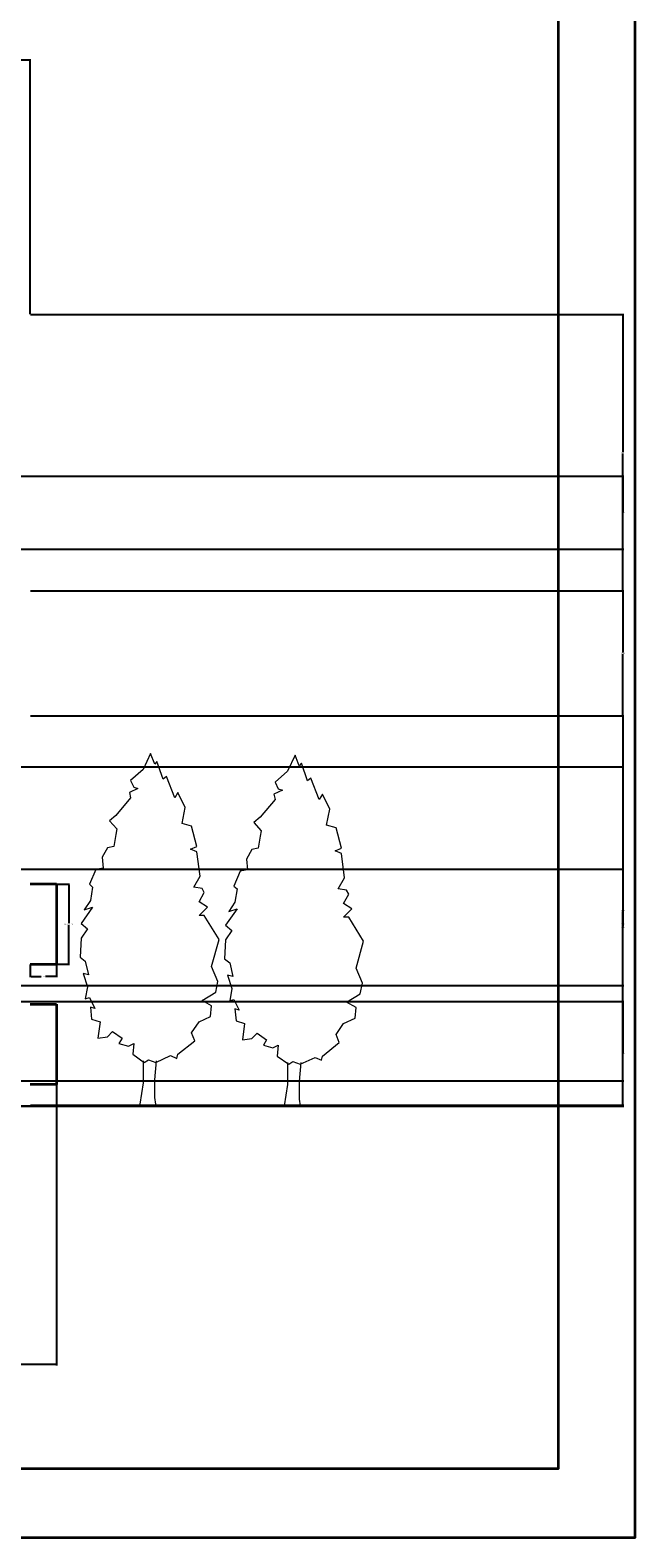
# Model space of a CAD drawing. Units: inches. Extents: x -279 to 364, y -385 to 335.
# Tile 4 of 9: x 238 to 364, y -385 to -72. Entities that reach past the tile are written whole.
import ezdxf

# ---------------------------------------------------------------- set-up
doc = ezdxf.new("R2010")
doc.units = ezdxf.units.IN
doc.header["$MEASUREMENT"] = 0
for name, color, linetype, lineweight in [('A-ANNO-DIMS', 2, 'Continuous', 18), ('A-ANNO-TTLB', 7, 'Continuous', 35), ('A-WALL', 7, 'Continuous', 35), ('C-TOPO', 32, 'Continuous', 30), ('L-PLNT', 94, 'Continuous', 13)]:
    doc.layers.add(name, color=color, linetype=linetype, lineweight=lineweight)
doc.styles.get("Standard").update_dxf_attribs({"font": 'arial.ttf'})
doc.dimstyles.get("Standard").update_dxf_attribs({"dimtxt": 0.18, "dimasz": 0.18, "dimexe": 0.18, "dimexo": 0.0625, "dimgap": 0.09, "dimtad": 0, "dimtih": 1, "dimtoh": 1, "dimdec": 4, "dimzin": 0, "dimdsep": 46, "dimtxsty": 'Standard', "dimcen": 0.09, "dimadec": 0, "dimazin": 0, "dimtfac": 1, "dimtdec": 4, "dimtofl": 0, "dimtmove": 0, "dimatfit": 3, "dimfxl": 1, "dimtolj": 1, "dimtzin": 0, "dimarcsym": 0})

# ---------------------------------------------------------------- blocks, each defined once
blk = doc.blocks.new('*U3')
blk.add_lwpolyline([(-2.754, 191.699), (-6.78, 182.851), (-13.682, 176.953), (-11.956, 173.266), (-9.656, 172.529), (-14.257, 170.317), (-13.682, 167.368), (-21.733, 157.783), (-25.184, 154.834), (-21.158, 150.41), (-21.733, 147.461), (-22.884, 140.825), (-26.334, 140.087), (-29.21, 134.926), (-28.635, 129.028), (-32.661, 128.291), (-36.111, 120.18), (-34.386, 118.706), (-35.536, 111.333), (-38.987, 106.171), (-34.386, 107.646), (-40.712, 98.798), (-37.261, 95.849), (-40.712, 90.688), (-41.287, 80.366), (-38.412, 78.154), (-36.686, 70.781), (-39.562, 71.518), (-37.261, 64.145), (-38.412, 57.509), (-36.111, 58.247), (-33.236, 52.348), (-35.536, 53.086), (-34.961, 46.45), (-30.36, 44.975), (-31.51, 36.128), (-26.334, 36.865), (-23.459, 39.814), (-18.283, 36.128), (-20.008, 33.178), (-14.832, 31.704), (-11.956, 33.178), (-12.531, 27.28), (-6.205, 22.856), (-3.905, 24.331), (0.121, 22.856), (8.173, 26.543), (11.624, 25.068), (12.199, 27.28), (21.4, 34.653), (19.675, 39.077), (23.701, 44.975), (30.027, 47.924), (30.602, 53.823), (25.426, 56.772), (32.903, 61.196), (34.053, 67.094), (30.602, 75.205), (34.628, 89.951), (26.576, 103.222), (23.701, 103.222), (28.302, 107.646), (23.701, 110.595), (26.576, 115.756), (25.426, 117.968), (20.825, 118.706), (24.276, 124.604), (22.551, 137.876), (19.1, 139.35), (22.551, 140.825), (19.675, 151.884), (14.499, 153.359), (16.224, 162.207), (12.199, 170.317), (10.473, 167.368), (5.872, 179.165), (4.147, 177.69), (0.696, 187.275), (-0.454, 185.8)], close=True)
for points in [[(-6.813, 23.669), (-6.813, 11.669), (-8.627, 0)], [(0.387, 23.669), (-0.576, 13.271), (-0.576, 3.686), (0, 0)]]:
    blk.add_lwpolyline(points)
blk = doc.blocks.new('PROJECTION-SIDE')
for p, q in [((0, 16.72), (5.49, 16.72)), ((5.49, 16.72), (5.49, 0)), ((5.49, 0), (0, 0))]:
    blk.add_line(p, q)
blk = doc.blocks.new('*D68')
at = {"layer": 'A-ANNO-DIMS', "color": 0, "lineweight": -2, "transparency": 16777216}
for p, q in [((243.89, -249.21), (246.52, -249.21)), ((246.34, -249.39), (246.34, -257.38)), ((246.34, -265.74), (246.34, -257.75)), ((243.89, -265.92), (246.52, -265.92))]:
    blk.add_line(p, q, dxfattribs=at)
at = {"layer": 'A-ANNO-DIMS', "color": 0, "transparency": 16777216}
for points in [[(246.31, -249.39), (246.37, -249.39), (246.34, -249.21)], [(246.31, -265.74), (246.37, -265.74), (246.34, -265.92)]]:
    blk.add_solid(points, dxfattribs=at)
at = {"layer": 'Defpoints', "color": 0, "transparency": 16777216}
for p in [(243.83, -249.21), (246.34, -249.21), (243.83, -265.92)]:
    blk.add_point(p, dxfattribs=at)
at = {"layer": 'A-ANNO-DIMS', "color": 0, "transparency": 16777216, "insert": (246.34, -257.56), "char_height": 0.18, "attachment_point": 5}
blk.add_mtext('\\A1;RETURN 17 TYP.', dxfattribs=at)
blk = doc.blocks.new('*D69')
at = {"layer": 'A-ANNO-DIMS', "color": 0, "lineweight": -2, "transparency": 16777216}
for p, q in [((238.34, -265.99), (238.34, -268.61)), ((243.83, -265.99), (243.83, -268.61)), ((238.52, -268.43), (240.62, -268.43)), ((243.65, -268.43), (241.54, -268.43))]:
    blk.add_line(p, q, dxfattribs=at)
at = {"layer": 'A-ANNO-DIMS', "color": 0, "transparency": 16777216}
for points in [[(238.52, -268.4), (238.52, -268.46), (238.34, -268.43)], [(243.65, -268.4), (243.65, -268.46), (243.83, -268.43)]]:
    blk.add_solid(points, dxfattribs=at)
at = {"layer": 'Defpoints', "color": 0, "transparency": 16777216}
for p in [(238.34, -265.92), (243.83, -265.92), (243.83, -268.43)]:
    blk.add_point(p, dxfattribs=at)
at = {"layer": 'A-ANNO-DIMS', "color": 0, "transparency": 16777216, "insert": (241.08, -268.43), "char_height": 0.18, "attachment_point": 5}
blk.add_mtext('\\A1;5 TYP.', dxfattribs=at)
blk = doc.blocks.new('*D97')
at = {"layer": 'A-ANNO-DIMS', "color": 0, "lineweight": -2, "transparency": 16777216}
for p, q in [((243.83, -291), (243.83, -349.37)), ((-125.57, -295.46), (-125.57, -349.37)), ((-125.39, -349.19), (58.74, -349.19)), ((243.65, -349.19), (59.52, -349.19))]:
    blk.add_line(p, q, dxfattribs=at)
at = {"layer": 'A-ANNO-DIMS', "color": 0, "transparency": 16777216}
for points in [[(-125.39, -349.16), (-125.39, -349.22), (-125.57, -349.19)], [(243.65, -349.16), (243.65, -349.22), (243.83, -349.19)]]:
    blk.add_solid(points, dxfattribs=at)
at = {"layer": 'Defpoints', "color": 0, "transparency": 16777216}
for p in [(243.83, -290.94), (-125.57, -295.4), (243.83, -349.19)]:
    blk.add_point(p, dxfattribs=at)
at = {"layer": 'A-ANNO-DIMS', "color": 0, "transparency": 16777216, "insert": (59.13, -349.19), "char_height": 0.18, "attachment_point": 5}
blk.add_mtext('\\A1;369.4', dxfattribs=at)
blk = doc.blocks.new('*D101')
at = {"layer": 'A-ANNO-DIMS', "color": 0, "lineweight": -2, "transparency": 16777216}
for p, q in [((114.35, -130.65), (114.35, -77.65)), ((114.53, -77.83), (176.06, -77.83)), ((238.16, -77.83), (176.62, -77.83)), ((238.34, -130.65), (238.34, -77.65))]:
    blk.add_line(p, q, dxfattribs=at)
at = {"layer": 'A-ANNO-DIMS', "color": 0, "transparency": 16777216}
for points in [[(114.53, -77.8), (114.53, -77.86), (114.35, -77.83)], [(238.16, -77.8), (238.16, -77.86), (238.34, -77.83)]]:
    blk.add_solid(points, dxfattribs=at)
at = {"layer": 'Defpoints', "color": 0, "transparency": 16777216}
for p in [(238.34, -77.83), (114.35, -130.71), (238.34, -130.71)]:
    blk.add_point(p, dxfattribs=at)
at = {"layer": 'A-ANNO-DIMS', "color": 0, "transparency": 16777216, "insert": (176.34, -77.83), "char_height": 0.18, "attachment_point": 5}
blk.add_mtext('\\A1;124', dxfattribs=at)
blk = doc.blocks.new('*D102')
at = {"layer": 'A-ANNO-DIMS', "color": 0, "lineweight": -2, "transparency": 16777216}
for p, q in [((238.4, -214.21), (361.74, -214.21)), ((361.56, -214.39), (361.56, -254.55)), ((361.56, -295.07), (361.56, -254.91)), ((238.4, -295.25), (361.74, -295.25))]:
    blk.add_line(p, q, dxfattribs=at)
at = {"layer": 'A-ANNO-DIMS', "color": 0, "transparency": 16777216}
for points in [[(361.53, -214.39), (361.59, -214.39), (361.56, -214.21)], [(361.53, -295.07), (361.59, -295.07), (361.56, -295.25)]]:
    blk.add_solid(points, dxfattribs=at)
at = {"layer": 'Defpoints', "color": 0, "transparency": 16777216}
for p in [(238.34, -214.21), (361.56, -214.21), (238.34, -295.25)]:
    blk.add_point(p, dxfattribs=at)
at = {"layer": 'A-ANNO-DIMS', "color": 0, "transparency": 16777216, "insert": (361.56, -254.73), "char_height": 0.18, "attachment_point": 5}
blk.add_mtext('\\A1;81.04', dxfattribs=at)
blk = doc.blocks.new('*D103')
at = {"layer": 'A-ANNO-DIMS', "color": 0, "lineweight": -2, "transparency": 16777216}
for p, q in [((238.4, -188.22), (361.74, -188.22)), ((361.56, -188.4), (361.56, -201.03)), ((361.56, -214.03), (361.56, -201.4)), ((238.4, -214.21), (361.74, -214.21))]:
    blk.add_line(p, q, dxfattribs=at)
at = {"layer": 'A-ANNO-DIMS', "color": 0, "transparency": 16777216}
for points in [[(361.53, -188.4), (361.59, -188.4), (361.56, -188.22)], [(361.53, -214.03), (361.59, -214.03), (361.56, -214.21)]]:
    blk.add_solid(points, dxfattribs=at)
at = {"layer": 'Defpoints', "color": 0, "transparency": 16777216}
for p in [(238.34, -188.22), (361.56, -188.22), (238.34, -214.21)]:
    blk.add_point(p, dxfattribs=at)
at = {"layer": 'A-ANNO-DIMS', "color": 0, "transparency": 16777216, "insert": (361.56, -201.21), "char_height": 0.18, "attachment_point": 5}
blk.add_mtext('\\A1;25.994', dxfattribs=at)
blk = doc.blocks.new('*D104')
at = {"layer": 'A-ANNO-DIMS', "color": 0, "lineweight": -2, "transparency": 16777216}
for p, q in [((238.4, -130.71), (361.74, -130.71)), ((361.56, -130.89), (361.56, -159.28)), ((361.56, -188.04), (361.56, -159.65)), ((238.4, -188.22), (361.74, -188.22))]:
    blk.add_line(p, q, dxfattribs=at)
at = {"layer": 'A-ANNO-DIMS', "color": 0, "transparency": 16777216}
for points in [[(361.53, -130.89), (361.59, -130.89), (361.56, -130.71)], [(361.53, -188.04), (361.59, -188.04), (361.56, -188.22)]]:
    blk.add_solid(points, dxfattribs=at)
at = {"layer": 'Defpoints', "color": 0, "transparency": 16777216}
for p in [(238.34, -130.71), (361.56, -130.71), (238.34, -188.22)]:
    blk.add_point(p, dxfattribs=at)
at = {"layer": 'A-ANNO-DIMS', "color": 0, "transparency": 16777216, "insert": (361.56, -159.47), "char_height": 0.18, "attachment_point": 5}
blk.add_mtext('\\A1;57.5', dxfattribs=at)
blk = doc.blocks.new('*D111')
at = {"layer": 'A-ANNO-DIMS', "color": 0, "lineweight": -2, "transparency": 16777216}
for p, q in [((184.08, -164.35), (361.74, -164.35)), ((361.56, -164.53), (361.56, -171.76)), ((361.56, -179.35), (361.56, -172.12)), ((184.92, -179.53), (361.74, -179.53))]:
    blk.add_line(p, q, dxfattribs=at)
at = {"layer": 'A-ANNO-DIMS', "color": 0, "transparency": 16777216}
for points in [[(361.53, -164.53), (361.59, -164.53), (361.56, -164.35)], [(361.53, -179.35), (361.59, -179.35), (361.56, -179.53)]]:
    blk.add_solid(points, dxfattribs=at)
at = {"layer": 'Defpoints', "color": 0, "transparency": 16777216}
for p in [(184.01, -164.35), (184.86, -179.53), (361.56, -179.53)]:
    blk.add_point(p, dxfattribs=at)
at = {"layer": 'A-ANNO-DIMS', "color": 0, "transparency": 16777216, "insert": (361.56, -171.94), "char_height": 0.18, "attachment_point": 5}
blk.add_mtext('\\A1;15.182', dxfattribs=at)
blk = doc.blocks.new('*D112')
at = {"layer": 'A-ANNO-DIMS', "color": 0, "lineweight": -2, "transparency": 16777216}
for p, q in [((177.91, -246.11), (361.74, -246.11)), ((361.56, -246.29), (361.56, -258.03)), ((361.56, -270.13), (361.56, -258.39)), ((177.91, -270.31), (361.74, -270.31))]:
    blk.add_line(p, q, dxfattribs=at)
at = {"layer": 'A-ANNO-DIMS', "color": 0, "transparency": 16777216}
for points in [[(361.53, -246.29), (361.59, -246.29), (361.56, -246.11)], [(361.53, -270.13), (361.59, -270.13), (361.56, -270.31)]]:
    blk.add_solid(points, dxfattribs=at)
at = {"layer": 'Defpoints', "color": 0, "transparency": 16777216}
for p in [(177.85, -246.11), (177.85, -270.31), (361.56, -270.31)]:
    blk.add_point(p, dxfattribs=at)
at = {"layer": 'A-ANNO-DIMS', "color": 0, "transparency": 16777216, "insert": (361.56, -258.21), "char_height": 0.18, "attachment_point": 5}
blk.add_mtext('\\A1;24.193', dxfattribs=at)
blk = doc.blocks.new('*D114')
at = {"layer": 'A-ANNO-DIMS', "color": 0, "lineweight": -2, "transparency": 16777216}
for p, q in [((222.66, -224.85), (361.74, -224.85)), ((361.56, -225.03), (361.56, -257.32)), ((361.56, -289.96), (361.56, -257.68)), ((222.66, -290.14), (361.74, -290.14))]:
    blk.add_line(p, q, dxfattribs=at)
at = {"layer": 'A-ANNO-DIMS', "color": 0, "transparency": 16777216}
for points in [[(361.53, -225.03), (361.59, -225.03), (361.56, -224.85)], [(361.53, -289.96), (361.59, -289.96), (361.56, -290.14)]]:
    blk.add_solid(points, dxfattribs=at)
at = {"layer": 'Defpoints', "color": 0, "transparency": 16777216}
for p in [(222.59, -224.85), (361.56, -224.85), (222.59, -290.14)]:
    blk.add_point(p, dxfattribs=at)
at = {"layer": 'A-ANNO-DIMS', "color": 0, "transparency": 16777216, "insert": (361.56, -257.5), "char_height": 0.18, "attachment_point": 5}
blk.add_mtext('\\A1;65.29', dxfattribs=at)
blk = doc.blocks.new('*D116')
at = {"layer": 'A-ANNO-DIMS', "color": 0, "lineweight": -2, "transparency": 16777216}
for p, q in [((78.52, -273.62), (361.74, -273.62)), ((361.56, -273.8), (361.56, -284.32)), ((361.56, -295.22), (361.56, -284.69)), ((78.52, -295.4), (361.74, -295.4))]:
    blk.add_line(p, q, dxfattribs=at)
at = {"layer": 'A-ANNO-DIMS', "color": 0, "transparency": 16777216}
for points in [[(361.53, -273.8), (361.59, -273.8), (361.56, -273.62)], [(361.53, -295.22), (361.59, -295.22), (361.56, -295.4)]]:
    blk.add_solid(points, dxfattribs=at)
at = {"layer": 'Defpoints', "color": 0, "transparency": 16777216}
for p in [(78.46, -273.62), (361.56, -273.62), (78.46, -295.4)]:
    blk.add_point(p, dxfattribs=at)
at = {"layer": 'A-ANNO-DIMS', "color": 0, "transparency": 16777216, "insert": (361.56, -284.51), "char_height": 0.18, "attachment_point": 5}
blk.add_mtext('\\A1;21.78', dxfattribs=at)

msp = doc.modelspace()

# ---------------------------------------------------------------- linework, layer by layer
at = {"layer": 'A-ANNO-TTLB'}
for points in [[(-279.2289, 334.6468), (364.0508, 334.6468), (364.0508, -385.2219), (-279.2289, -385.2219)], [(-267.2403, 317.5778), (348.1051, 317.5778), (348.1051, -370.8321), (-267.2403, -370.8321)]]:
    msp.add_lwpolyline(points, close=True, dxfattribs=at)
at = {"layer": 'C-TOPO'}
for p, q in [((195.2296, -295.3951), (256.846, -295.3951)), ((256.846, -295.3951), (282.224, -295.3951)), ((282.224, -295.3951), (335.1088, -295.3951))]:
    msp.add_line(p, q, dxfattribs=at)

# ---------------------------------------------------------------- block references
at = {"layer": 'A-WALL'}
for p in [(238.336, -265.924), (238.336, -290.941)]:
    msp.add_blockref('PROJECTION-SIDE', p, dxfattribs=at)
at = {"layer": 'L-PLNT', "xscale": 0.3806743271777806, "yscale": 0.3806743271777806, "zscale": 0.3806743271777806}
for p in [(264.418, -295.0231), (294.4493, -295.376)]:
    msp.add_blockref('*U3', p, dxfattribs=at)

# ---------------------------------------------------------------- dimensions: what is measured, and where the dimension line sits
at = {"layer": 'A-ANNO-DIMS'}
for base, p1, p2, override, picture, middle in [((238.3359, -77.8255), (114.3455, -130.7132), (238.3359, -130.7132), {"dimdec": 0, "dimlfac": 1, "dimrnd": 0, "dimzin": 0, "dimdsep": 46, "dimlunit": 2}, '*D101', (176.3407, -77.8255)), ((243.8297, -349.1915), (-125.5669, -295.3951), (243.8297, -290.9407), {"dimdec": 1, "dimlfac": 1, "dimrnd": 0, "dimzin": 0, "dimdsep": 46, "dimlunit": 2}, '*D97', (59.1314, -349.1915))]:
    dim = msp.add_linear_dim(base=base, p1=p1, p2=p2, dimstyle='Standard', override=override, dxfattribs=at)
    dim.commit()
    dim.dimension.update_dxf_attribs({"geometry": picture, "text_midpoint": middle})
for base, p1, p2, override, picture, middle in [((361.5588, -130.7132), (238.3359, -188.2171), (238.3359, -130.7132), {"dimdec": 1, "dimlfac": 1, "dimrnd": 0, "dimzin": 0, "dimdsep": 46, "dimlunit": 2}, '*D104', (361.5588, -159.4652)), ((361.55885, -179.53263), (184.013, -164.35109), (184.85741, -179.53263), {"dimdec": 3, "dimlfac": 1, "dimrnd": 0, "dimzin": 0, "dimdsep": 46, "dimlunit": 2}, '*D111', (361.55885, -171.94186)), ((361.5588, -188.2171), (238.3359, -214.2107), (238.3359, -188.2171), {"dimdec": 3, "dimlfac": 1, "dimrnd": 0, "dimzin": 0, "dimdsep": 46, "dimlunit": 2}, '*D103', (361.5588, -201.2139)), ((361.5588, -214.2107), (238.3359, -295.2473), (238.3359, -214.2107), {"dimdec": 2, "dimlfac": 1, "dimrnd": 0, "dimzin": 0, "dimdsep": 46, "dimlunit": 2}, '*D102', (361.5588, -254.729)), ((361.5588, -224.8549), (222.5949, -290.1425), (222.5949, -224.8549), {"dimdec": 2, "dimlfac": 1, "dimrnd": 0, "dimzin": 0, "dimdsep": 46, "dimlunit": 2}, '*D114', (361.5588, -257.4987)), ((361.5588, -270.3054), (177.8517, -246.1124), (177.8517, -270.3054), {"dimdec": 3, "dimlfac": 1, "dimrnd": 0, "dimzin": 0, "dimdsep": 46, "dimlunit": 2}, '*D112', (361.5588, -258.2089)), ((361.5588, -273.6155), (78.4572, -295.3951), (78.4572, -273.6155), {"dimdec": 2, "dimlfac": 1, "dimrnd": 0, "dimzin": 0, "dimdsep": 46, "dimlunit": 2}, '*D116', (361.5588, -284.5053))]:
    dim = msp.add_linear_dim(base=base, p1=p1, p2=p2, angle=90, dimstyle='Standard', override=override, dxfattribs=at)
    dim.commit()
    dim.dimension.update_dxf_attribs({"geometry": picture, "text_midpoint": middle})
dim = msp.add_linear_dim(base=(246.3374, -249.2055), p1=(243.8297, -265.9237), p2=(243.8297, -249.2055), angle=90, text='RETURN <> TYP.', dimstyle='Standard', override={"dimdec": 0, "dimlfac": 1, "dimrnd": 0, "dimzin": 0, "dimdsep": 46, "dimlunit": 2}, dxfattribs=at)
dim.commit()
dim.dimension.update_dxf_attribs({"geometry": '*D68', "text_midpoint": (246.3374, -257.5646)})
dim = msp.add_linear_dim(base=(243.8297, -268.4314), p1=(238.3359, -265.9237), p2=(243.8297, -265.9237), text='<> TYP.', dimstyle='Standard', override={"dimdec": 0, "dimlfac": 1, "dimrnd": 0, "dimzin": 0, "dimdsep": 46, "dimlunit": 2}, dxfattribs=at)
dim.commit()
dim.dimension.update_dxf_attribs({"geometry": '*D69', "text_midpoint": (241.0828, -268.4314)})

doc.saveas('drawing.dxf')
